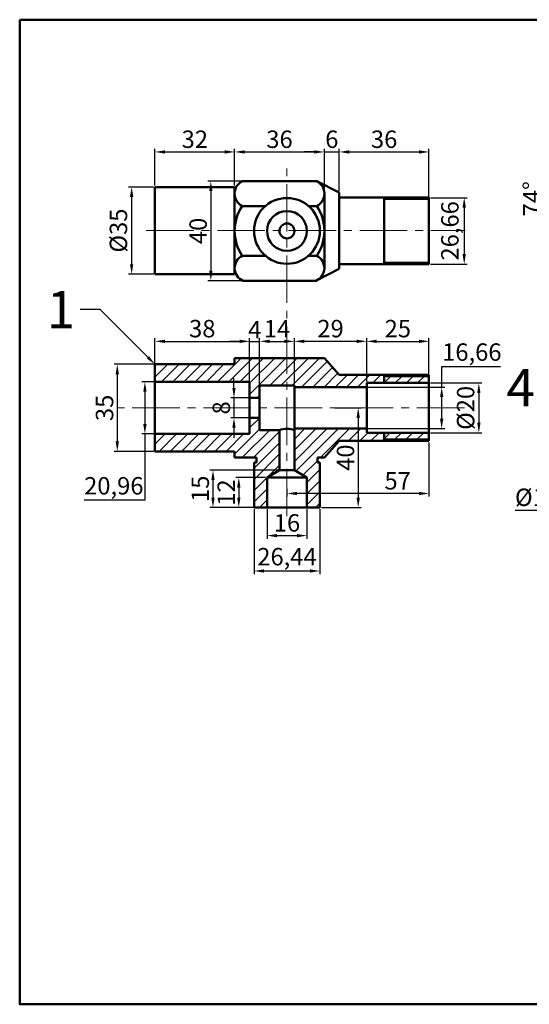
# Model space of a CAD drawing. Units: millimetres. Extents: x 123 to 731, y 468 to 864.
# Tile 1 of 5: x 123 to 328, y 468 to 864. Entities that reach past the tile are written whole.
import ezdxf
from ezdxf import colors
from ezdxf.entities.mleader import LeaderData, LeaderLine
from ezdxf.math import Vec2, Vec3

# ---------------------------------------------------------------- set-up
doc = ezdxf.new("R2010")
doc.units = ezdxf.units.MM
doc.linetypes.add('CENTER2', pattern=[28.575, 19.05, -3.175, 3.175, -3.175])
for name, color, linetype, lineweight in [('M-CNTR', 1, 'CENTER2', 18), ('M-DIMS', 2, 'Continuous', 25), ('M-HATC', 8, 'Continuous', 18), ('M-OUTL', 7, 'Continuous', 50), ('M-TEXT', 3, 'Continuous', 25)]:
    doc.layers.add(name, color=color, linetype=linetype, lineweight=lineweight)
doc.styles.get("Standard").update_dxf_attribs({"font": 'arial.ttf'})
doc.dimstyles.new('ISO-25', dxfattribs={"dimtxt": 7, "dimasz": 4, "dimexe": 1.25, "dimexo": 0.625, "dimtad": 1, "dimtoh": 1, "dimtxsty": 'Standard', "dimcen": 2.5, "dimadec": 0, "dimazin": 0, "dimtfac": 1, "dimtmove": 0, "dimatfit": 3, "dimfxl": 1, "dimarcsym": 0})

# ---------------------------------------------------------------- blocks, each defined once
blk = doc.blocks.new('*U1')
at = {"layer": 'M-CNTR', "color": 0, "transparency": 16777216}
blk.add_line((0, -14.93), (0, 124.78), dxfattribs=at)
blk = doc.blocks.new('*U2')
at = {"layer": 'M-CNTR', "color": 0, "transparency": 16777216}
blk.add_line((105.24, 0), (-34.13, 0), dxfattribs=at)
blk = doc.blocks.new('*U3')
at = {"layer": 'M-CNTR', "color": 0, "transparency": 16777216}
blk.add_line((-19.5, 0), (108.55, 0), dxfattribs=at)
blk = doc.blocks.new('*D4')
at = {"layer": 'Defpoints', "color": 0, "transparency": 16777216}
for p in [(177.67, 796.75), (168.31, 761.75), (177.67, 761.75)]:
    blk.add_point(p, dxfattribs=at)
at = {"layer": 'M-DIMS', "color": 0, "lineweight": -2, "transparency": 16777216}
for p, q in [((177.04, 796.75), (167.06, 796.75)), ((168.31, 792.75), (168.31, 765.75)), ((177.04, 761.75), (167.06, 761.75))]:
    blk.add_line(p, q, dxfattribs=at)
at = {"layer": 'M-DIMS', "color": 0, "transparency": 16777216}
for points in [[(167.64, 792.75), (168.98, 792.75), (168.31, 796.75)], [(167.64, 765.75), (168.98, 765.75), (168.31, 761.75)]]:
    blk.add_solid(points, dxfattribs=at)
at = {"layer": 'M-DIMS', "color": 0, "transparency": 16777216, "insert": (163.91, 779.25), "char_height": 7, "attachment_point": 5, "rotation": 90}
blk.add_mtext('%%C35', dxfattribs=at)
blk = doc.blocks.new('*D5')
at = {"layer": 'Defpoints', "color": 0, "transparency": 16777216}
for p in [(209.67, 810.83), (177.67, 796.75), (209.67, 796.75)]:
    blk.add_point(p, dxfattribs=at)
at = {"layer": 'M-DIMS', "color": 0, "lineweight": -2, "transparency": 16777216}
for p, q in [((177.67, 797.38), (177.67, 812.08)), ((181.67, 810.83), (205.67, 810.83)), ((209.67, 797.38), (209.67, 812.08))]:
    blk.add_line(p, q, dxfattribs=at)
at = {"layer": 'M-DIMS', "color": 0, "transparency": 16777216}
for points in [[(181.67, 811.5), (181.67, 810.17), (177.67, 810.83)], [(205.67, 811.5), (205.67, 810.17), (209.67, 810.83)]]:
    blk.add_solid(points, dxfattribs=at)
at = {"layer": 'M-DIMS', "color": 0, "transparency": 16777216, "insert": (193.67, 815.03), "char_height": 7, "attachment_point": 5}
blk.add_mtext('32', dxfattribs=at)
blk = doc.blocks.new('*D6')
at = {"layer": 'Defpoints', "color": 0, "transparency": 16777216}
for p in [(245.67, 810.83), (209.67, 800.51), (245.67, 789.41)]:
    blk.add_point(p, dxfattribs=at)
at = {"layer": 'M-DIMS', "color": 0, "lineweight": -2, "transparency": 16777216}
for p, q in [((209.67, 801.14), (209.67, 812.08)), ((213.67, 810.83), (241.67, 810.83)), ((245.67, 790.04), (245.67, 812.08))]:
    blk.add_line(p, q, dxfattribs=at)
at = {"layer": 'M-DIMS', "color": 0, "transparency": 16777216}
for points in [[(213.67, 811.5), (213.67, 810.17), (209.67, 810.83)], [(241.67, 811.5), (241.67, 810.17), (245.67, 810.83)]]:
    blk.add_solid(points, dxfattribs=at)
at = {"layer": 'M-DIMS', "color": 0, "transparency": 16777216, "insert": (227.67, 815.03), "char_height": 7, "attachment_point": 5}
blk.add_mtext('36', dxfattribs=at)
blk = doc.blocks.new('*D7')
at = {"layer": 'Defpoints', "color": 0, "transparency": 16777216}
for p in [(287.67, 810.83), (251.67, 794.59), (287.67, 791.97)]:
    blk.add_point(p, dxfattribs=at)
at = {"layer": 'M-DIMS', "color": 0, "lineweight": -2, "transparency": 16777216}
for p, q in [((251.67, 795.22), (251.67, 812.08)), ((255.67, 810.83), (283.67, 810.83)), ((287.67, 792.6), (287.67, 812.08))]:
    blk.add_line(p, q, dxfattribs=at)
at = {"layer": 'M-DIMS', "color": 0, "transparency": 16777216}
for points in [[(255.67, 811.5), (255.67, 810.17), (251.67, 810.83)], [(283.67, 811.5), (283.67, 810.17), (287.67, 810.83)]]:
    blk.add_solid(points, dxfattribs=at)
at = {"layer": 'M-DIMS', "color": 0, "transparency": 16777216, "insert": (269.67, 815.03), "char_height": 7, "attachment_point": 5}
blk.add_mtext('36', dxfattribs=at)
blk = doc.blocks.new('*D8')
at = {"layer": 'Defpoints', "color": 0, "transparency": 16777216}
for p in [(287.67, 792.47), (287.67, 765.81), (301.82, 765.81)]:
    blk.add_point(p, dxfattribs=at)
at = {"layer": 'M-DIMS', "color": 0, "lineweight": -2, "transparency": 16777216}
for p, q in [((288.29, 792.47), (303.07, 792.47)), ((301.82, 788.47), (301.82, 769.81)), ((288.29, 765.81), (303.07, 765.81))]:
    blk.add_line(p, q, dxfattribs=at)
at = {"layer": 'M-DIMS', "color": 0, "transparency": 16777216}
for points in [[(301.15, 788.47), (302.49, 788.47), (301.82, 792.47)], [(301.15, 769.81), (302.49, 769.81), (301.82, 765.81)]]:
    blk.add_solid(points, dxfattribs=at)
at = {"layer": 'M-DIMS', "color": 0, "transparency": 16777216, "insert": (296.99, 779.14), "char_height": 7, "attachment_point": 5, "rotation": 90}
blk.add_mtext('26,66', dxfattribs=at)
blk = doc.blocks.new('*D9')
at = {"layer": 'Defpoints', "color": 0, "transparency": 16777216}
for p in [(217.45, 799.11), (200.1, 759.11), (217.45, 759.11)]:
    blk.add_point(p, dxfattribs=at)
at = {"layer": 'M-DIMS', "color": 0, "lineweight": -2, "transparency": 16777216}
for p, q in [((216.83, 799.11), (198.85, 799.11)), ((200.1, 795.11), (200.1, 763.11)), ((216.83, 759.11), (198.85, 759.11))]:
    blk.add_line(p, q, dxfattribs=at)
at = {"layer": 'M-DIMS', "color": 0, "transparency": 16777216}
for points in [[(199.43, 795.11), (200.76, 795.11), (200.1, 799.11)], [(199.43, 763.11), (200.76, 763.11), (200.1, 759.11)]]:
    blk.add_solid(points, dxfattribs=at)
at = {"layer": 'M-DIMS', "color": 0, "transparency": 16777216, "insert": (195.9, 779.11), "char_height": 7, "attachment_point": 5, "rotation": 90}
blk.add_mtext('40', dxfattribs=at)
blk = doc.blocks.new('*D10')
at = {"layer": 'Defpoints', "color": 0, "transparency": 16777216}
for p in [(215.67, 734.76), (177.67, 718.51), (215.67, 718.51)]:
    blk.add_point(p, dxfattribs=at)
at = {"layer": 'M-DIMS', "color": 0, "lineweight": -2, "transparency": 16777216}
for p, q in [((177.67, 719.14), (177.67, 736.01)), ((215.67, 719.14), (215.67, 736.01)), ((181.67, 734.76), (211.67, 734.76))]:
    blk.add_line(p, q, dxfattribs=at)
at = {"layer": 'M-DIMS', "color": 0, "transparency": 16777216}
for points in [[(181.67, 735.43), (181.67, 734.09), (177.67, 734.76)], [(211.67, 735.43), (211.67, 734.09), (215.67, 734.76)]]:
    blk.add_solid(points, dxfattribs=at)
at = {"layer": 'M-DIMS', "color": 0, "transparency": 16777216, "insert": (196.67, 738.96), "char_height": 7, "attachment_point": 5}
blk.add_mtext('38', dxfattribs=at)
blk = doc.blocks.new('*D11')
at = {"layer": 'Defpoints', "color": 0, "transparency": 16777216}
for p in [(219.67, 734.76), (215.67, 712.03), (219.67, 712.03)]:
    blk.add_point(p, dxfattribs=at)
at = {"layer": 'M-DIMS', "color": 0, "lineweight": -2, "transparency": 16777216}
for p, q in [((215.67, 712.66), (215.67, 736.01)), ((219.67, 712.66), (219.67, 736.01)), ((211.67, 734.76), (207.67, 734.76)), ((215.67, 734.76), (219.67, 734.76)), ((223.67, 734.76), (227.67, 734.76))]:
    blk.add_line(p, q, dxfattribs=at)
at = {"layer": 'M-DIMS', "color": 0, "transparency": 16777216}
for points in [[(211.67, 735.43), (211.67, 734.09), (215.67, 734.76)], [(223.67, 735.43), (223.67, 734.09), (219.67, 734.76)]]:
    blk.add_solid(points, dxfattribs=at)
at = {"layer": 'M-DIMS', "color": 0, "transparency": 16777216, "insert": (217.72, 738.51), "char_height": 7, "attachment_point": 5}
blk.add_mtext('4', dxfattribs=at)
blk = doc.blocks.new('*D12')
at = {"layer": 'Defpoints', "color": 0, "transparency": 16777216}
for p in [(233.67, 734.76), (219.67, 717), (233.67, 717)]:
    blk.add_point(p, dxfattribs=at)
at = {"layer": 'M-DIMS', "color": 0, "lineweight": -2, "transparency": 16777216}
for p, q in [((219.67, 717.62), (219.67, 736.01)), ((233.67, 717.62), (233.67, 736.01)), ((223.67, 734.76), (229.67, 734.76))]:
    blk.add_line(p, q, dxfattribs=at)
at = {"layer": 'M-DIMS', "color": 0, "transparency": 16777216}
for points in [[(223.67, 735.43), (223.67, 734.09), (219.67, 734.76)], [(229.67, 735.43), (229.67, 734.09), (233.67, 734.76)]]:
    blk.add_solid(points, dxfattribs=at)
at = {"layer": 'M-DIMS', "color": 0, "transparency": 16777216, "insert": (226.67, 738.9), "char_height": 7, "attachment_point": 5}
blk.add_mtext('14', dxfattribs=at)
blk = doc.blocks.new('*D13')
at = {"layer": 'Defpoints', "color": 0, "transparency": 16777216}
for p in [(233.67, 734.76), (233.67, 718.03), (262.67, 718.03)]:
    blk.add_point(p, dxfattribs=at)
at = {"layer": 'M-DIMS', "color": 0, "lineweight": -2, "transparency": 16777216}
for p, q in [((233.67, 718.66), (233.67, 736.01)), ((262.67, 718.66), (262.67, 736.01)), ((258.67, 734.76), (237.67, 734.76))]:
    blk.add_line(p, q, dxfattribs=at)
at = {"layer": 'M-DIMS', "color": 0, "transparency": 16777216}
for points in [[(237.67, 735.43), (237.67, 734.09), (233.67, 734.76)], [(258.67, 735.43), (258.67, 734.09), (262.67, 734.76)]]:
    blk.add_solid(points, dxfattribs=at)
at = {"layer": 'M-DIMS', "color": 0, "transparency": 16777216, "insert": (248.17, 738.96), "char_height": 7, "attachment_point": 5}
blk.add_mtext('29', dxfattribs=at)
blk = doc.blocks.new('*D14')
at = {"layer": 'Defpoints', "color": 0, "transparency": 16777216}
for p in [(287.67, 734.76), (262.67, 721.25), (287.67, 721.25)]:
    blk.add_point(p, dxfattribs=at)
at = {"layer": 'M-DIMS', "color": 0, "lineweight": -2, "transparency": 16777216}
for p, q in [((262.67, 721.88), (262.67, 736.01)), ((287.67, 721.88), (287.67, 736.01)), ((266.67, 734.76), (283.67, 734.76))]:
    blk.add_line(p, q, dxfattribs=at)
at = {"layer": 'M-DIMS', "color": 0, "transparency": 16777216}
for points in [[(266.67, 735.43), (266.67, 734.09), (262.67, 734.76)], [(283.67, 735.43), (283.67, 734.09), (287.67, 734.76)]]:
    blk.add_solid(points, dxfattribs=at)
at = {"layer": 'M-DIMS', "color": 0, "transparency": 16777216, "insert": (275.17, 738.96), "char_height": 7, "attachment_point": 5}
blk.add_mtext('25', dxfattribs=at)
blk = doc.blocks.new('*D15')
at = {"layer": 'Defpoints', "color": 0, "transparency": 16777216}
for p in [(262.67, 716.36), (262.67, 699.7), (292.78, 699.7)]:
    blk.add_point(p, dxfattribs=at)
at = {"layer": 'M-DIMS', "color": 0, "lineweight": -2, "transparency": 16777216}
for p, q in [((292.78, 716.36), (292.78, 724.7)), ((292.78, 724.7), (316.36, 724.7)), ((263.29, 716.36), (294.03, 716.36)), ((292.78, 703.7), (292.78, 712.36)), ((263.29, 699.7), (294.03, 699.7))]:
    blk.add_line(p, q, dxfattribs=at)
at = {"layer": 'M-DIMS', "color": 0, "transparency": 16777216}
for points in [[(292.11, 712.36), (293.45, 712.36), (292.78, 716.36)], [(292.11, 703.7), (293.45, 703.7), (292.78, 699.7)]]:
    blk.add_solid(points, dxfattribs=at)
at = {"layer": 'M-DIMS', "color": 0, "transparency": 16777216, "insert": (304.88, 729.53), "char_height": 7, "attachment_point": 5}
blk.add_mtext('16,66', dxfattribs=at)
blk = doc.blocks.new('*D16')
at = {"layer": 'Defpoints', "color": 0, "transparency": 16777216}
for p in [(287.67, 718.03), (287.67, 698.03), (307.7, 698.03)]:
    blk.add_point(p, dxfattribs=at)
at = {"layer": 'M-DIMS', "color": 0, "lineweight": -2, "transparency": 16777216}
for p, q in [((288.29, 718.03), (308.95, 718.03)), ((307.7, 714.03), (307.7, 702.03)), ((288.29, 698.03), (308.95, 698.03))]:
    blk.add_line(p, q, dxfattribs=at)
at = {"layer": 'M-DIMS', "color": 0, "transparency": 16777216}
for points in [[(307.03, 714.03), (308.37, 714.03), (307.7, 718.03)], [(307.03, 702.03), (308.37, 702.03), (307.7, 698.03)]]:
    blk.add_solid(points, dxfattribs=at)
at = {"layer": 'M-DIMS', "color": 0, "transparency": 16777216, "insert": (303.31, 708.03), "char_height": 7, "attachment_point": 5, "rotation": 90}
blk.add_mtext('%%C20', dxfattribs=at)
blk = doc.blocks.new('*D17')
at = {"layer": 'Defpoints', "color": 0, "transparency": 16777216}
for p in [(249.32, 708.03), (243.89, 668.03), (259.27, 668.03)]:
    blk.add_point(p, dxfattribs=at)
at = {"layer": 'M-DIMS', "color": 0, "lineweight": -2, "transparency": 16777216}
for p, q in [((249.94, 708.03), (260.52, 708.03)), ((259.27, 704.03), (259.27, 672.03)), ((244.51, 668.03), (260.52, 668.03))]:
    blk.add_line(p, q, dxfattribs=at)
at = {"layer": 'M-DIMS', "color": 0, "transparency": 16777216}
for points in [[(258.6, 704.03), (259.93, 704.03), (259.27, 708.03)], [(258.6, 672.03), (259.93, 672.03), (259.27, 668.03)]]:
    blk.add_solid(points, dxfattribs=at)
at = {"layer": 'M-DIMS', "color": 0, "transparency": 16777216, "insert": (255.07, 688.03), "char_height": 7, "attachment_point": 5, "rotation": 90}
blk.add_mtext('40', dxfattribs=at)
blk = doc.blocks.new('*D18')
at = {"layer": 'Defpoints', "color": 0, "transparency": 16777216}
for p in [(222.67, 680.03), (211.34, 668.03), (222.67, 668.03)]:
    blk.add_point(p, dxfattribs=at)
at = {"layer": 'M-DIMS', "color": 0, "lineweight": -2, "transparency": 16777216}
for p, q in [((222.04, 680.03), (210.09, 680.03)), ((211.34, 676.03), (211.34, 672.03)), ((222.04, 668.03), (210.09, 668.03))]:
    blk.add_line(p, q, dxfattribs=at)
at = {"layer": 'M-DIMS', "color": 0, "transparency": 16777216}
for points in [[(210.67, 676.03), (212.01, 676.03), (211.34, 680.03)], [(210.67, 672.03), (212.01, 672.03), (211.34, 668.03)]]:
    blk.add_solid(points, dxfattribs=at)
at = {"layer": 'M-DIMS', "color": 0, "transparency": 16777216, "insert": (207.2, 674.03), "char_height": 7, "attachment_point": 5, "rotation": 90}
blk.add_mtext('12', dxfattribs=at)
blk = doc.blocks.new('*D19')
at = {"layer": 'Defpoints', "color": 0, "transparency": 16777216}
for p in [(227.67, 683.03), (200.96, 668.03), (227.67, 668.03)]:
    blk.add_point(p, dxfattribs=at)
at = {"layer": 'M-DIMS', "color": 0, "lineweight": -2, "transparency": 16777216}
for p, q in [((227.04, 683.03), (199.71, 683.03)), ((200.96, 679.03), (200.96, 672.03)), ((227.04, 668.03), (199.71, 668.03))]:
    blk.add_line(p, q, dxfattribs=at)
at = {"layer": 'M-DIMS', "color": 0, "transparency": 16777216}
for points in [[(200.29, 679.03), (201.62, 679.03), (200.96, 683.03)], [(200.29, 672.03), (201.62, 672.03), (200.96, 668.03)]]:
    blk.add_solid(points, dxfattribs=at)
at = {"layer": 'M-DIMS', "color": 0, "transparency": 16777216, "insert": (196.76, 675.53), "char_height": 7, "attachment_point": 5, "rotation": 90}
blk.add_mtext('15', dxfattribs=at)
blk = doc.blocks.new('*D20')
at = {"layer": 'Defpoints', "color": 0, "transparency": 16777216}
for p in [(222.67, 668.03), (238.67, 668.03), (238.67, 656.72)]:
    blk.add_point(p, dxfattribs=at)
at = {"layer": 'M-DIMS', "color": 0, "lineweight": -2, "transparency": 16777216}
for p, q in [((222.67, 667.41), (222.67, 655.47)), ((238.67, 667.41), (238.67, 655.47)), ((226.67, 656.72), (234.67, 656.72))]:
    blk.add_line(p, q, dxfattribs=at)
at = {"layer": 'M-DIMS', "color": 0, "transparency": 16777216}
for points in [[(226.67, 657.38), (226.67, 656.05), (222.67, 656.72)], [(234.67, 657.38), (234.67, 656.05), (238.67, 656.72)]]:
    blk.add_solid(points, dxfattribs=at)
at = {"layer": 'M-DIMS', "color": 0, "transparency": 16777216, "insert": (230.67, 660.92), "char_height": 7, "attachment_point": 5}
blk.add_mtext('16', dxfattribs=at)
blk = doc.blocks.new('*D21')
at = {"layer": 'Defpoints', "color": 0, "transparency": 16777216}
for p in [(217.45, 668.03), (243.89, 668.03), (243.89, 642.51)]:
    blk.add_point(p, dxfattribs=at)
at = {"layer": 'M-DIMS', "color": 0, "lineweight": -2, "transparency": 16777216}
for p, q in [((217.45, 667.41), (217.45, 641.26)), ((243.89, 667.41), (243.89, 641.26)), ((221.45, 642.51), (239.89, 642.51))]:
    blk.add_line(p, q, dxfattribs=at)
at = {"layer": 'M-DIMS', "color": 0, "transparency": 16777216}
for points in [[(221.45, 643.18), (221.45, 641.85), (217.45, 642.51)], [(239.89, 643.18), (239.89, 641.85), (243.89, 642.51)]]:
    blk.add_solid(points, dxfattribs=at)
at = {"layer": 'M-DIMS', "color": 0, "transparency": 16777216, "insert": (230.67, 647.35), "char_height": 7, "attachment_point": 5}
blk.add_mtext('26,44', dxfattribs=at)
blk = doc.blocks.new('*D22')
at = {"layer": 'Defpoints', "color": 0, "transparency": 16777216}
for p in [(287.67, 694.81), (230.67, 676.07), (230.67, 673.64)]:
    blk.add_point(p, dxfattribs=at)
at = {"layer": 'M-DIMS', "color": 0, "lineweight": -2, "transparency": 16777216}
for p, q in [((287.67, 694.19), (287.67, 672.39)), ((230.67, 675.45), (230.67, 672.39)), ((283.67, 673.64), (234.67, 673.64))]:
    blk.add_line(p, q, dxfattribs=at)
at = {"layer": 'M-DIMS', "color": 0, "transparency": 16777216}
for points in [[(234.67, 674.31), (234.67, 672.98), (230.67, 673.64)], [(283.67, 674.31), (283.67, 672.98), (287.67, 673.64)]]:
    blk.add_solid(points, dxfattribs=at)
at = {"layer": 'M-DIMS', "color": 0, "transparency": 16777216, "insert": (275.11, 677.83), "char_height": 7, "attachment_point": 5}
blk.add_mtext('57', dxfattribs=at)
blk = doc.blocks.new('*D23')
at = {"layer": 'Defpoints', "color": 0, "transparency": 16777216}
for p in [(215.67, 712.03), (209.4, 704.03), (215.67, 704.03)]:
    blk.add_point(p, dxfattribs=at)
at = {"layer": 'M-DIMS', "color": 0, "lineweight": -2, "transparency": 16777216}
for p, q in [((209.4, 716.03), (209.4, 720.03)), ((215.04, 712.03), (208.15, 712.03)), ((209.4, 712.03), (209.4, 704.03)), ((215.04, 704.03), (208.15, 704.03)), ((209.4, 700.03), (209.4, 696.03))]:
    blk.add_line(p, q, dxfattribs=at)
at = {"layer": 'M-DIMS', "color": 0, "transparency": 16777216}
for points in [[(208.73, 716.03), (210.06, 716.03), (209.4, 712.03)], [(208.73, 700.03), (210.06, 700.03), (209.4, 704.03)]]:
    blk.add_solid(points, dxfattribs=at)
at = {"layer": 'M-DIMS', "color": 0, "transparency": 16777216, "insert": (205.2, 708.03), "char_height": 7, "attachment_point": 5, "rotation": 90}
blk.add_mtext('8', dxfattribs=at)
blk = doc.blocks.new('*D24')
at = {"layer": 'Defpoints', "color": 0, "transparency": 16777216}
for p in [(177.67, 718.51), (173.64, 697.55), (177.67, 697.55)]:
    blk.add_point(p, dxfattribs=at)
at = {"layer": 'M-DIMS', "color": 0, "lineweight": -2, "transparency": 16777216}
for p, q in [((177.04, 718.51), (172.39, 718.51)), ((173.64, 714.51), (173.64, 701.55)), ((177.04, 697.55), (172.39, 697.55)), ((173.64, 697.55), (173.64, 671)), ((173.64, 671), (149.28, 671))]:
    blk.add_line(p, q, dxfattribs=at)
at = {"layer": 'M-DIMS', "color": 0, "transparency": 16777216}
for points in [[(172.97, 714.51), (174.31, 714.51), (173.64, 718.51)], [(172.97, 701.55), (174.31, 701.55), (173.64, 697.55)]]:
    blk.add_solid(points, dxfattribs=at)
at = {"layer": 'M-DIMS', "color": 0, "transparency": 16777216, "insert": (161.15, 675.83), "char_height": 7, "attachment_point": 5}
blk.add_mtext('20,96', dxfattribs=at)
blk = doc.blocks.new('*D25')
at = {"layer": 'Defpoints', "color": 0, "transparency": 16777216}
for p in [(177.67, 725.53), (162.54, 690.53), (177.67, 690.53)]:
    blk.add_point(p, dxfattribs=at)
at = {"layer": 'M-DIMS', "color": 0, "lineweight": -2, "transparency": 16777216}
for p, q in [((177.04, 725.53), (161.29, 725.53)), ((162.54, 721.53), (162.54, 694.53)), ((177.04, 690.53), (161.29, 690.53))]:
    blk.add_line(p, q, dxfattribs=at)
at = {"layer": 'M-DIMS', "color": 0, "transparency": 16777216}
for points in [[(161.88, 721.53), (163.21, 721.53), (162.54, 725.53)], [(161.88, 694.53), (163.21, 694.53), (162.54, 690.53)]]:
    blk.add_solid(points, dxfattribs=at)
at = {"layer": 'M-DIMS', "color": 0, "transparency": 16777216, "insert": (158.34, 708.03), "char_height": 7, "attachment_point": 5, "rotation": 90}
blk.add_mtext('35', dxfattribs=at)
blk = doc.blocks.new('*D28')
at = {"layer": 'Defpoints', "color": 0, "transparency": 16777216}
for p in [(355.16, 798.03), (334.32, 794.85), (350.16, 794.26), (350.16, 789.8), (355.16, 786.03)]:
    blk.add_point(p, dxfattribs=at)
at = {"layer": 'M-DIMS', "color": 0, "lineweight": -2, "transparency": 16777216}
for p, q in [((346.7, 792.41), (335.67, 800.72)), ((346.7, 791.65), (335.67, 783.34))]:
    blk.add_line(p, q, dxfattribs=at)
for start, end in [(108.0972, 125.5486), (143, 217), (234.4514, 251.9028)]:
    blk.add_arc((347.2, 792.03), 13.18, start, end, dxfattribs=at)
at = {"layer": 'M-DIMS', "color": 0, "transparency": 16777216}
for points in [[(340, 802.28), (339.07, 803.23), (336.67, 799.97)], [(339.07, 780.83), (340, 781.78), (336.67, 784.1)]]:
    blk.add_solid(points, dxfattribs=at)
at = {"layer": 'M-DIMS', "color": 0, "transparency": 16777216, "insert": (329.89, 792.03), "char_height": 7, "attachment_point": 5, "rotation": 90}
blk.add_mtext('74°', dxfattribs=at)
blk = doc.blocks.new('*D73')
at = {"layer": 'Defpoints', "color": 0, "transparency": 16777216}
for p in [(351.93, 688.82), (340.5, 670.82), (351.93, 670.82)]:
    blk.add_point(p, dxfattribs=at)
at = {"layer": 'M-DIMS', "color": 0, "lineweight": -2, "transparency": 16777216}
for p, q in [((351.31, 688.82), (339.25, 688.82)), ((340.5, 684.82), (340.5, 674.82)), ((351.31, 670.82), (339.25, 670.82)), ((340.5, 670.82), (340.5, 666.82)), ((340.5, 666.82), (322.22, 666.82))]:
    blk.add_line(p, q, dxfattribs=at)
at = {"layer": 'M-DIMS', "color": 0, "transparency": 16777216}
for points in [[(339.83, 684.82), (341.17, 684.82), (340.5, 688.82)], [(339.83, 674.82), (341.17, 674.82), (340.5, 670.82)]]:
    blk.add_solid(points, dxfattribs=at)
at = {"layer": 'M-DIMS', "color": 0, "transparency": 16777216, "insert": (331.05, 671.21), "char_height": 7, "attachment_point": 5}
blk.add_mtext('%%C18', dxfattribs=at)
blk = doc.blocks.new('*D81')
at = {"layer": 'Defpoints', "color": 0, "transparency": 16777216}
for p in [(245.67, 810.83), (251.67, 810.83), (251.67, 810.83)]:
    blk.add_point(p, dxfattribs=at)
at = {"layer": 'M-DIMS', "color": 0, "lineweight": -2, "transparency": 16777216}
for p, q in [((241.67, 810.83), (237.67, 810.83)), ((245.67, 811.46), (245.67, 812.08)), ((245.67, 810.83), (251.67, 810.83)), ((251.67, 811.46), (251.67, 812.08)), ((255.67, 810.83), (259.67, 810.83))]:
    blk.add_line(p, q, dxfattribs=at)
at = {"layer": 'M-DIMS', "color": 0, "transparency": 16777216}
for points in [[(241.67, 811.5), (241.67, 810.17), (245.67, 810.83)], [(255.67, 811.5), (255.67, 810.17), (251.67, 810.83)]]:
    blk.add_solid(points, dxfattribs=at)
at = {"layer": 'M-DIMS', "color": 0, "transparency": 16777216, "insert": (248.67, 815.03), "char_height": 7, "attachment_point": 5}
blk.add_mtext('6', dxfattribs=at)

msp = doc.modelspace()

# ---------------------------------------------------------------- hatches: boundary and pattern name
at = {"layer": 'M-HATC'}
h = msp.add_hatch(dxfattribs=at)
h.set_pattern_fill('ANSI31', color=256)
h.set_pattern_definition([(45, (-17.5532, 552.0506), (-2.245064, 2.245064), [])])
h.paths.add_polyline_path([(230.6696, 728.0323), (209.6696, 728.0323), (209.6696, 725.5323), (177.6696, 725.5323), (177.6696, 718.5123), (215.6696, 718.5123), (215.6696, 712.0323), (219.6696, 712.0323), (219.6696, 716.9952), (230.6696, 716.9952)])
h.paths.add_polyline_path([(245.6696, 728.0323), (230.6696, 728.0323), (230.6696, 716.9952), (233.6696, 716.9952), (233.6696, 716.3623), (262.6696, 716.3623), (262.6696, 718.0323), (269.6696, 718.0323), (269.6696, 721.2523), (262.6696, 721.2523), (251.6696, 721.2523)])
h.paths.add_polyline_path([(227.6696, 699.0694), (219.6696, 699.0694), (219.6696, 704.0323), (215.6696, 704.0323), (215.6696, 697.5523), (177.6696, 697.5523), (177.6696, 690.5323), (209.6696, 690.5323), (209.6696, 688.0323), (218.4496, 688.0323), (218.4496, 686.0323), (217.4496, 686.0323), (217.4496, 668.0323), (222.6696, 668.0323), (222.6696, 680.0323), (227.6696, 683.0323)])
h.paths.add_polyline_path([(251.6696, 694.8123), (262.6696, 694.8123), (269.6696, 694.8123), (269.6696, 698.0323), (262.6696, 698.0323), (262.6696, 699.7023), (233.6696, 699.7023), (233.6696, 699.0694), (233.6696, 683.0323), (238.6696, 680.0323), (238.6696, 668.0323), (243.8896, 668.0323), (243.8896, 686.0323), (242.8896, 686.0323), (242.8896, 688.0323), (245.6696, 688.0323)])
h.paths.add_polyline_path([(287.6696, 698.0323), (269.6696, 698.0323), (269.6696, 695.3123), (287.6696, 695.3123)])
h.paths.add_polyline_path([(287.6696, 720.7523), (269.6696, 720.7523), (269.6696, 718.0323), (287.6696, 718.0323)])

# ---------------------------------------------------------------- linework, layer by layer
at = {"layer": 'M-OUTL'}
for p, q in [((242.6696, 799.1135), (212.6696, 799.1135)), ((242.6696, 799.1135), (251.6696, 794.5921)), ((177.6696, 761.7547), (177.6696, 796.7547)), ((177.6696, 796.7547), (209.6696, 796.7547)), ((209.6696, 796.7547), (209.6696, 761.7547)), ((209.6696, 794.5921), (209.6696, 763.9173)), ((245.6696, 763.9173), (245.6696, 794.5921)), ((251.6696, 763.9173), (251.6696, 794.5921)), ((251.6696, 779.2547), (251.6696, 792.4747)), ((251.6696, 792.4747), (287.6696, 792.4747)), ((269.6696, 792.4747), (269.6696, 765.8147)), ((269.6696, 791.9747), (287.6696, 791.9747)), ((287.6696, 792.4747), (287.6696, 765.8147)), ((212.6696, 789.1135), (222.0227, 789.1135)), ((239.3165, 789.1135), (242.6696, 789.1135)), ((212.6696, 769.1135), (222.0227, 769.1135)), ((239.3165, 769.1135), (242.6696, 769.1135)), ((242.2736, 759.1135), (251.6696, 763.9173)), ((287.6696, 765.8147), (251.6696, 765.8147)), ((287.6696, 766.3147), (269.6696, 766.3147)), ((209.6696, 761.7547), (177.6696, 761.7547)), ((213.0656, 759.1135), (242.2736, 759.1135)), ((209.6696, 725.5323), (209.6696, 728.0323)), ((209.6696, 728.0323), (245.6696, 728.0323)), ((251.6696, 721.2523), (245.6696, 728.0323)), ((177.6696, 725.5323), (177.6696, 718.5123)), ((177.6696, 725.5323), (209.6696, 725.5323)), ((262.6696, 721.2523), (251.6696, 721.2523)), ((287.6696, 721.2523), (262.6696, 721.2523)), ((269.6696, 721.2523), (269.6696, 718.0323)), ((269.6696, 720.7523), (287.6696, 720.7523)), ((287.6696, 708.0323), (287.6696, 721.2523)), ((215.6696, 718.5123), (177.6696, 718.5123)), ((177.6696, 718.5123), (177.6696, 697.5523)), ((215.6696, 718.5123), (215.6696, 712.0323)), ((219.6696, 716.9952), (219.6696, 699.0694)), ((233.6696, 716.9952), (219.6696, 716.9952)), ((233.6696, 716.9952), (233.6696, 708.0323)), ((262.6696, 716.3623), (233.6696, 716.3623)), ((233.6696, 708.0323), (233.6696, 716.3623)), ((262.6696, 718.0323), (262.6696, 698.0323)), ((287.6696, 718.0323), (262.6696, 718.0323)), ((287.6696, 718.0323), (287.6696, 694.8123)), ((219.6696, 712.0323), (215.6696, 712.0323)), ((215.6696, 712.0323), (215.6696, 704.0323)), ((219.6696, 712.0323), (219.6696, 704.0323)), ((233.6696, 708.0323), (233.6696, 699.7023)), ((233.6696, 699.0694), (233.6696, 708.0323)), ((215.6696, 704.0323), (219.6696, 704.0323)), ((215.6696, 697.5523), (215.6696, 704.0323)), ((177.6696, 697.5523), (215.6696, 697.5523)), ((177.6696, 690.5323), (177.6696, 697.5523)), ((227.6696, 699.0694), (219.6696, 699.0694)), ((227.6696, 699.0694), (227.6696, 683.0323)), ((262.6696, 699.7023), (233.6696, 699.7023)), ((233.6696, 699.0694), (233.6696, 683.0323)), ((287.6696, 698.0323), (262.6696, 698.0323)), ((269.6696, 698.0323), (269.6696, 694.8123)), ((251.6696, 694.8123), (245.6696, 688.0323)), ((262.6696, 694.8123), (251.6696, 694.8123)), ((287.6696, 694.8123), (262.6696, 694.8123)), ((287.6696, 694.8123), (262.6696, 694.8123)), ((269.6696, 695.3123), (287.6696, 695.3123)), ((177.6696, 690.5323), (209.6696, 690.5323)), ((209.6696, 690.5323), (209.6696, 688.0323)), ((209.6696, 688.0323), (218.4496, 688.0323)), ((217.4496, 688.0323), (218.4496, 688.0323)), ((217.4496, 668.0323), (217.4496, 686.0323)), ((218.4496, 686.0323), (217.4496, 686.0323)), ((218.4496, 688.0323), (218.4496, 686.0323)), ((242.8896, 688.0323), (242.8896, 686.0323)), ((242.8896, 688.0323), (245.6696, 688.0323)), ((242.8896, 686.0323), (243.8896, 686.0323)), ((243.8896, 668.0323), (243.8896, 686.0323)), ((227.6696, 683.0323), (222.6696, 680.0323)), ((227.6696, 683.0323), (233.6696, 683.0323)), ((233.6696, 683.0323), (238.6696, 680.0323)), ((238.6696, 680.0323), (222.6696, 680.0323)), ((222.6696, 680.0323), (222.6696, 668.0323)), ((238.6696, 668.0323), (238.6696, 680.0323)), ((230.6696, 668.0323), (217.4496, 668.0323)), ((222.6696, 668.0323), (238.6696, 668.0323)), ((230.6696, 668.0323), (243.8896, 668.0323))]:
    msp.add_line(p, q, dxfattribs=at)
msp.add_lwpolyline([(123.3719, 863.9604), (731.4761, 863.9604), (731.4761, 468.4518), (123.3719, 468.4518)], close=True, dxfattribs=at)
for radius in [13.22, 8, 3]:
    msp.add_circle((230.6696, 779.1135), radius, dxfattribs=at)
for centre, radius, start, end in [((215.2981, 794.1135), 5.6488, 117.730707, 242.269293), ((240.0411, 794.1135), 5.6488, 297.730707, 62.269293), ((227.8363, 779.1135), 18.1667, 146.601512, 213.398488), ((227.5029, 779.1135), 18.1667, 326.601512, 33.398488), ((215.1718, 764.2047), 5.5097, 117.010017, 247.525168), ((240.1674, 764.2047), 5.5097, 292.474832, 62.989983), ((230.6696, 691.5243), 8.1196, 68.316751, 111.683249)]:
    msp.add_arc(centre, radius, start, end, dxfattribs=at)

# ---------------------------------------------------------------- block references
at = {"layer": 'M-CNTR'}
for name, p in [('*U1', (230.6696, 679.4582)), ('*U3', (193.6696, 779.2547)), ('*U2', (196.6696, 708.0323))]:
    msp.add_blockref(name, p, dxfattribs=at)

# ---------------------------------------------------------------- dimensions: what is measured, and where the dimension line sits
at = {"layer": 'M-DIMS'}
for base, p1, p2, picture, middle in [((209.6696, 810.8327), (177.6696, 796.7547), (209.6696, 796.7547), '*D5', (193.6696, 815.0341)), ((245.6696, 810.8327), (209.6696, 800.513), (245.6696, 789.4125), '*D6', (227.6696, 815.0341)), ((251.6696, 810.8327), (245.6696, 810.8327), (251.6696, 810.8327), '*D81', (248.6696, 815.0317)), ((287.6696, 810.8327), (251.6696, 794.5921), (287.6696, 791.9747), '*D7', (269.6696, 815.0341)), ((215.6696, 734.7593), (177.6696, 718.5123), (215.6696, 718.5123), '*D10', (196.6696, 738.9607)), ((233.6696, 734.7593), (219.6696, 716.9952), (233.6696, 716.9952), '*D12', (226.6696, 738.8987)), ((233.6696, 734.7593), (262.6696, 718.0323), (233.6696, 718.0323), '*D13', (248.1696, 738.9583)), ((287.6696, 734.7593), (262.6696, 721.2523), (287.6696, 721.2523), '*D14', (275.1696, 738.9583)), ((243.8896, 642.5137), (217.4496, 668.0323), (243.8896, 668.0323), '*D21', (230.6696, 647.3454)), ((238.6696, 656.7168), (222.6696, 668.0323), (238.6696, 668.0323), '*D20', (230.6696, 660.9158))]:
    dim = msp.add_linear_dim(base=base, p1=p1, p2=p2, dimstyle='ISO-25', override={"dimclrd": 0, "dimclre": 0, "dimclrt": 0}, dxfattribs=at)
    dim.commit()
    dim.dimension.update_dxf_attribs({"geometry": picture, "text_midpoint": middle})
dim = msp.add_angular_dim_2l(base=(334.3166, 794.8471), line1=((350.1582, 789.7989), (355.1582, 786.0311)), line2=((355.1582, 798.0311), (350.1582, 794.2634)), dimstyle='ISO-25', override={"dimclrd": 0, "dimclre": 0, "dimclrt": 0}, dxfattribs=at)
dim.commit()
dim.dimension.update_dxf_attribs({"geometry": '*D28', "text_midpoint": (329.8874, 792.0311)})
for base, p1, p2, picture, middle in [((200.0953, 759.1135), (217.4529, 799.1135), (217.4529, 759.1135), '*D9', (195.8963, 779.1135)), ((301.8214, 765.8147), (287.6696, 792.4747), (287.6696, 765.8147), '*D8', (296.9897, 779.1447)), ((209.3953, 704.0323), (215.6696, 712.0323), (215.6696, 704.0323), '*D23', (205.1962, 708.0323)), ((259.2668, 668.0323), (249.3191, 708.0323), (243.8896, 668.0323), '*D17', (255.0678, 688.0323)), ((200.9579, 668.0323), (227.6696, 683.0323), (227.6696, 668.0323), '*D19', (196.7589, 675.5323)), ((211.3412, 668.0323), (222.6696, 680.0323), (222.6696, 668.0323), '*D18', (207.2019, 674.0323))]:
    dim = msp.add_linear_dim(base=base, p1=p1, p2=p2, angle=90, dimstyle='ISO-25', override={"dimclrd": 0, "dimclre": 0, "dimclrt": 0}, dxfattribs=at)
    dim.commit()
    dim.dimension.update_dxf_attribs({"geometry": picture, "text_midpoint": middle})
for base, p1, p2, picture, middle in [((168.3096, 761.7547), (177.6696, 796.7547), (177.6696, 761.7547), '*D4', (163.9148, 779.2547)), ((307.7006, 698.0323), (287.6696, 718.0323), (287.6696, 698.0323), '*D16', (303.3059, 708.0323)), ((340.5007, 670.8159), (351.9314, 688.8159), (351.9314, 670.8159), '*D73', (331.0469, 671.2107))]:
    dim = msp.add_linear_dim(base=base, p1=p1, p2=p2, angle=90, text='%%C<>', dimstyle='ISO-25', override={"dimclrd": 0, "dimclre": 0, "dimclrt": 0}, dxfattribs=at)
    dim.commit()
    dim.dimension.update_dxf_attribs({"geometry": picture, "text_midpoint": middle})
for base, p1, p2, picture, middle in [((219.6696, 734.7593), (215.6696, 712.0323), (219.6696, 712.0323), '*D11', (217.723, 738.5093)), ((230.6696, 673.6424), (287.6696, 694.8123), (230.6696, 676.0743), '*D22', (275.114, 677.8271))]:
    dim = msp.add_linear_dim(base=base, p1=p1, p2=p2, dimstyle='ISO-25', override={"dimclrd": 0, "dimclre": 0, "dimclrt": 0, "dimtmove": 2}, dxfattribs=at)
    dim.commit()
    dim.dimension.update_dxf_attribs({"geometry": picture, "text_midpoint": middle, "dimtype": 160})
for base, p1, p2, picture, middle in [((292.7789, 699.7023), (262.6696, 716.3623), (262.6696, 699.7023), '*D15', (304.8827, 724.6977)), ((162.5446, 690.5323), (177.6696, 725.5323), (177.6696, 690.5323), '*D25', (162.5446, 708.0323)), ((173.6413, 697.5523), (177.6696, 718.5123), (177.6696, 697.5523), '*D24', (161.1483, 671.003))]:
    dim = msp.add_linear_dim(base=base, p1=p1, p2=p2, angle=90, dimstyle='ISO-25', override={"dimclrd": 0, "dimclre": 0, "dimclrt": 0}, dxfattribs=at)
    dim.commit()
    dim.dimension.update_dxf_attribs({"geometry": picture, "text_midpoint": middle, "dimtype": 160})

# ---------------------------------------------------------------- leaders
at = {"layer": 'M-TEXT'}
ml = msp.add_multileader_mtext('Standard', dxfattribs=at)
ml.set_content('1', color=256)
ml.set_leader_properties()
ml.build(insert=Vec2(0, 0))
ctx = ml.context
ctx.base_point, ctx.char_height, ctx.plane_origin = Vec3(138.0869, 747.4912), 15, Vec3(177.6696, 725.5323)
ctx.text_align_type = 2
notes = []
notes.append((ctx, [(0, (1, 1, 0), (155.6121, 747.4912), (-1, 0), 8, [(0, [(177.6696, 725.5323)], 0, [])])]))
ctx.mtext.insert, ctx.mtext.alignment, ctx.mtext.flow_direction = Vec3(145.6121, 754.9912), 3, 5
ml = msp.add_multileader_mtext('Standard', dxfattribs=at)
ml.set_content('4', color=256)
ml.set_leader_properties()
ml.build(insert=Vec2(0, 0))
ctx = ml.context
ctx.base_point, ctx.char_height, ctx.plane_origin = Vec3(317.7754, 716.1847), 15, Vec3(345.3205, 725.1393)
ctx.text_align_type = 2
notes.append((ctx, [(0, (1, 1, 0), (340.1506, 716.1847), (-1, 0), 8, [(0, [(345.3205, 725.1393)], 0, [])])]))
ctx.mtext.insert, ctx.mtext.alignment, ctx.mtext.flow_direction = Vec3(330.1506, 723.6847), 3, 5
for ctx, leaders in notes:
    for number, flags, end, landing, length, lines in leaders:
        leader = LeaderData()
        leader.index, (leader.has_last_leader_line, leader.has_dogleg_vector, leader.attachment_direction) = number, flags
        leader.last_leader_point, leader.dogleg_vector, leader.dogleg_length = Vec3(end), Vec3(landing), length
        for number, points, colour, breaks in lines:
            line = LeaderLine()
            line.index, line.vertices, line.color, line.breaks = number, Vec3.list(points), colors.encode_raw_color(colour), breaks
            leader.lines.append(line)
        ctx.leaders.append(leader)

doc.saveas('drawing.dxf')
